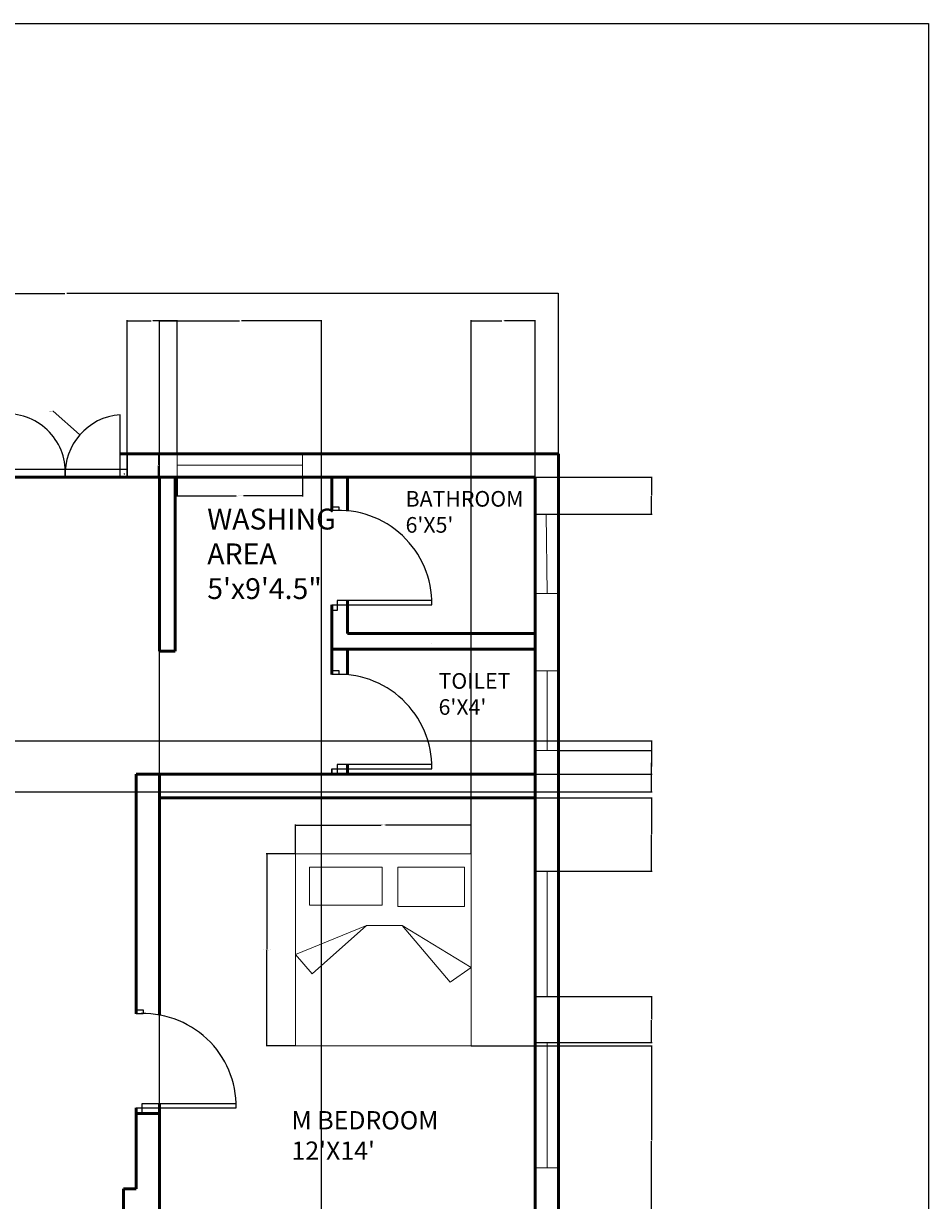
# Model space of a CAD drawing. Units: inches. Extents: x -177 to 2564, y -706 to 2548.
# Tile 4 of 4: x 176 to 523, y -266 to 186. Entities that reach past the tile are written whole.
import ezdxf

# ---------------------------------------------------------------- set-up
doc = ezdxf.new("R2010")
doc.units = ezdxf.units.IN
doc.header["$MEASUREMENT"] = 0
for name, color, linetype, lineweight in [('A-ANNO-DIMS', 2, 'Continuous', 18), ('A-ANNO-TTLB', 7, 'Continuous', 25), ('A-AREA-IDEN', 7, 'Continuous', 25), ('A-DOOR', 3, 'Continuous', 25), ('A-FURN', 8, 'Continuous', 18), ('A-GLAZ', 4, 'Continuous', 18), ('A-WALL', 7, 'Continuous', 50)]:
    doc.layers.add(name, color=color, linetype=linetype, lineweight=lineweight)
doc.styles.get("Standard").update_dxf_attribs({"font": 'arial.ttf'})
doc.dimstyles.get("Standard").update_dxf_attribs({"dimtxt": 0.18, "dimasz": 0.18, "dimexe": 0.18, "dimexo": 0.0625, "dimgap": 0.09, "dimtad": 0, "dimtih": 1, "dimtoh": 1, "dimdec": 0, "dimzin": 0, "dimdsep": 46, "dimlunit": 4, "dimtxsty": 'Standard', "dimcen": 0.09, "dimadec": 0, "dimazin": 0, "dimtfac": 1, "dimtdec": 0, "dimtofl": 0, "dimtmove": 0, "dimatfit": 3, "dimfxl": 1, "dimtolj": 1, "dimtzin": 0, "dimarcsym": 0})

# ---------------------------------------------------------------- blocks, each defined once
blk = doc.blocks.new('*D1')
at = {"layer": 'A-ANNO-DIMS', "color": 0, "lineweight": -2, "transparency": 16777216}
for p, q in [((3.47, 20.6), (3.47, 82.15)), ((3.65, 81.97), (192.07, 81.97)), ((381.29, 81.97), (192.87, 81.97)), ((381.47, 20.6), (381.47, 82.15))]:
    blk.add_line(p, q, dxfattribs=at)
at = {"layer": 'A-ANNO-DIMS', "color": 0, "transparency": 16777216}
for points in [[(3.65, 82), (3.65, 81.94), (3.47, 81.97)], [(381.29, 82), (381.29, 81.94), (381.47, 81.97)]]:
    blk.add_solid(points, dxfattribs=at)
at = {"layer": 'Defpoints', "color": 0, "transparency": 16777216}
for p in [(381.47, 81.97), (3.47, 20.54), (381.47, 20.54)]:
    blk.add_point(p, dxfattribs=at)
at = {"layer": 'A-ANNO-DIMS', "color": 0, "transparency": 16777216, "insert": (192.47, 81.97), "char_height": 0.18, "attachment_point": 5}
blk.add_mtext('\\A1;31\'-6"', dxfattribs=at)
blk = doc.blocks.new('BED-DOUBLE')
for p, q in [((0, -38.58), (27.19, -27.51)), ((27.19, -27.51), (6.3, -46)), ((27.19, -27.51), (40.92, -27.51)), ((40.92, -27.51), (27.19, -27.51)), ((40.92, -27.51), (67.3, -43.62)), ((59.29, -49.22), (40.92, -27.51)), ((0, -73.65), (0, -38.58)), ((6.3, -46), (0, -38.58)), ((67.3, -43.62), (59.29, -49.22))]:
    blk.add_line(p, q)
for points in [[(0, 0), (67.3, 0), (67.3, -73.65), (0, -73.65)], [(5.32, -5.1), (33.21, -5.1), (33.21, -19.67), (5.32, -19.67)], [(39.24, -5.1), (64.75, -5.1), (64.75, -20.23), (39.24, -20.23)]]:
    blk.add_lwpolyline(points, close=True)
blk = doc.blocks.new('WIN-48')
for p, q in [((0, 0), (9, 0)), ((9, 0), (4.59, 0)), ((4.59, 0), (4.59, -48.06)), ((9, -48.06), (0, -48.06))]:
    blk.add_line(p, q)
blk = doc.blocks.new('WIN-30')
for p, q in [((0, 30.54), (-9, 30.54)), ((-4.41, 0), (-4.41, 30.54)), ((0, 0), (-9, 0)), ((0, 0), (-4.41, 0))]:
    blk.add_line(p, q)
blk = doc.blocks.new('DOOR-SINGLE-36')
for p, q in [((1.57, 36.24), (0, 36.24)), ((0, 36.24), (0, 0)), ((1.57, -2.14), (1.57, 36.24)), ((1.57, 36.24), (1.57, 36.24)), ((-36.05, -2.14), (-36.05, 0.59)), ((-36.05, 0.59), (-34.54, 0.59)), ((-34.54, 0.59), (-34.54, -2.14)), ((0, 0), (3.72, 0)), ((3.72, 0), (3.72, -2.14)), ((3.72, -2.14), (1.57, -2.14))]:
    blk.add_line(p, q)
blk.add_arc((1.05, 0.56), 35.69, 89.1597, 184.3396)
blk = doc.blocks.new('DOOR-PAIR-44')
for p, q in [((0, 0), (0, 24.32)), ((44.01, 0), (44.01, 23.95)), ((-2.88, 0), (-2.88, 3.11)), ((-2.88, 3.11), (46.72, 3.11)), ((46.72, 0), (-2.88, 0)), ((-2.88, 0), (0, 0)), ((0, 0), (44.01, 0)), ((23.01, 0), (23.01, 3.55)), ((44.01, 0), (23.01, 0)), ((46.72, 0), (44.01, 0))]:
    blk.add_line(p, q)
for centre, radius, start, end in [((0.52, 1.77), 22.55, 355.4915, 91.326), ((45.7, 1.28), 22.73, 94.2755, 183.2347)]:
    blk.add_arc(centre, radius, start, end)
blk = doc.blocks.new('*D10')
at = {"layer": 'A-ANNO-DIMS', "color": 0, "lineweight": -2, "transparency": 16777216}
for p, q in [((235.2, 11.47), (235.2, 4.15)), ((283.26, 11.47), (283.26, 4.15)), ((235.38, 4.33), (257.78, 4.33)), ((283.08, 4.33), (260.68, 4.33))]:
    blk.add_line(p, q, dxfattribs=at)
at = {"layer": 'A-ANNO-DIMS', "color": 0, "transparency": 16777216}
for points in [[(235.38, 4.36), (235.38, 4.3), (235.2, 4.33)], [(283.08, 4.36), (283.08, 4.3), (283.26, 4.33)]]:
    blk.add_solid(points, dxfattribs=at)
at = {"layer": 'Defpoints', "color": 0, "transparency": 16777216}
for p in [(235.2, 11.54), (283.26, 11.54), (235.2, 4.33)]:
    blk.add_point(p, dxfattribs=at)
at = {"layer": 'A-ANNO-DIMS', "color": 0, "transparency": 16777216, "insert": (259.23, 4.33), "char_height": 0.18, "attachment_point": 5}
blk.add_mtext('\\A1;WINDOW W1 4\'-0" TYP.', dxfattribs=at)
blk = doc.blocks.new('*D11')
at = {"layer": 'A-ANNO-DIMS', "color": 0, "lineweight": -2, "transparency": 16777216}
for p, q in [((235.14, 20.54), (227.81, 20.54)), ((227.99, 20.36), (227.99, 16.22)), ((227.99, 11.72), (227.99, 15.85)), ((235.14, 11.54), (227.81, 11.54))]:
    blk.add_line(p, q, dxfattribs=at)
at = {"layer": 'A-ANNO-DIMS', "color": 0, "transparency": 16777216}
for points in [[(227.96, 20.36), (228.02, 20.36), (227.99, 20.54)], [(227.96, 11.72), (228.02, 11.72), (227.99, 11.54)]]:
    blk.add_solid(points, dxfattribs=at)
at = {"layer": 'Defpoints', "color": 0, "transparency": 16777216}
for p in [(227.99, 20.54), (235.2, 20.54), (235.2, 11.54)]:
    blk.add_point(p, dxfattribs=at)
at = {"layer": 'A-ANNO-DIMS', "color": 0, "transparency": 16777216, "insert": (227.99, 16.04), "char_height": 0.18, "attachment_point": 5}
blk.add_mtext('\\A1;0\'-9" TYP.', dxfattribs=at)
blk = doc.blocks.new('*D14')
at = {"layer": 'A-ANNO-DIMS', "color": 0, "lineweight": -2, "transparency": 16777216}
for p, q in [((280.56, -132.99), (269.4, -132.99)), ((269.58, -133.17), (269.58, -169.63)), ((269.58, -206.45), (269.58, -169.99)), ((280.56, -206.63), (269.4, -206.63))]:
    blk.add_line(p, q, dxfattribs=at)
at = {"layer": 'A-ANNO-DIMS', "color": 0, "transparency": 16777216}
for points in [[(269.55, -133.17), (269.61, -133.17), (269.58, -132.99)], [(269.55, -206.45), (269.61, -206.45), (269.58, -206.63)]]:
    blk.add_solid(points, dxfattribs=at)
at = {"layer": 'Defpoints', "color": 0, "transparency": 16777216}
for p in [(269.58, -132.99), (280.63, -132.99), (280.63, -206.63)]:
    blk.add_point(p, dxfattribs=at)
at = {"layer": 'A-ANNO-DIMS', "color": 0, "transparency": 16777216, "insert": (269.58, -169.81), "char_height": 0.18, "attachment_point": 5}
blk.add_mtext('\\A1;DOUBLE BED 6\'-1 1/2" TYP.', dxfattribs=at)
blk = doc.blocks.new('*D15')
at = {"layer": 'A-ANNO-DIMS', "color": 0, "lineweight": -2, "transparency": 16777216}
for p, q in [((280.63, -132.92), (280.63, -121.76)), ((347.93, -132.92), (347.93, -121.76)), ((280.81, -121.94), (313.43, -121.94)), ((347.75, -121.94), (315.13, -121.94))]:
    blk.add_line(p, q, dxfattribs=at)
at = {"layer": 'A-ANNO-DIMS', "color": 0, "transparency": 16777216}
for points in [[(280.81, -121.91), (280.81, -121.97), (280.63, -121.94)], [(347.75, -121.91), (347.75, -121.97), (347.93, -121.94)]]:
    blk.add_solid(points, dxfattribs=at)
at = {"layer": 'Defpoints', "color": 0, "transparency": 16777216}
for p in [(347.93, -121.94), (280.63, -132.99), (347.93, -132.99)]:
    blk.add_point(p, dxfattribs=at)
at = {"layer": 'A-ANNO-DIMS', "color": 0, "transparency": 16777216, "insert": (314.28, -121.94), "char_height": 0.18, "attachment_point": 5}
blk.add_mtext('\\A1;5\'-7 1/2" TYP.', dxfattribs=at)
blk = doc.blocks.new('*D36')
at = {"layer": 'A-ANNO-DIMS', "color": 0, "lineweight": -2, "transparency": 16777216}
for p, q in [((41.71, -89.59), (417.35, -89.59)), ((417.17, -89.77), (417.17, -99.17)), ((417.17, -108.95), (417.17, -99.54)), ((41.71, -109.13), (417.35, -109.13))]:
    blk.add_line(p, q, dxfattribs=at)
at = {"layer": 'A-ANNO-DIMS', "color": 0, "transparency": 16777216}
for points in [[(417.14, -89.77), (417.2, -89.77), (417.17, -89.59)], [(417.14, -108.95), (417.2, -108.95), (417.17, -109.13)]]:
    blk.add_solid(points, dxfattribs=at)
at = {"layer": 'Defpoints', "color": 0, "transparency": 16777216}
for p in [(41.65, -89.59), (41.65, -109.13), (417.17, -109.13)]:
    blk.add_point(p, dxfattribs=at)
at = {"layer": 'A-ANNO-DIMS', "color": 0, "transparency": 16777216, "insert": (417.17, -99.36), "char_height": 0.18, "attachment_point": 5}
blk.add_mtext('\\A1;1\'-7 1/2"', dxfattribs=at)
blk = doc.blocks.new('*D44')
at = {"layer": 'A-ANNO-DIMS', "color": 0, "lineweight": -2, "transparency": 16777216}
for p, q in [((372.54, -111.46), (417.35, -111.46)), ((417.17, -111.64), (417.17, -125.39)), ((417.17, -139.49), (417.17, -125.75)), ((372.54, -139.67), (417.35, -139.67))]:
    blk.add_line(p, q, dxfattribs=at)
at = {"layer": 'A-ANNO-DIMS', "color": 0, "transparency": 16777216}
for points in [[(417.14, -111.64), (417.2, -111.64), (417.17, -111.46)], [(417.14, -139.49), (417.2, -139.49), (417.17, -139.67)]]:
    blk.add_solid(points, dxfattribs=at)
at = {"layer": 'Defpoints', "color": 0, "transparency": 16777216}
for p in [(372.47, -111.46), (372.47, -139.67), (417.17, -139.67)]:
    blk.add_point(p, dxfattribs=at)
at = {"layer": 'A-ANNO-DIMS', "color": 0, "transparency": 16777216, "insert": (417.17, -125.57), "char_height": 0.18, "attachment_point": 5}
blk.add_mtext('\\A1;2\'-4"', dxfattribs=at)
blk = doc.blocks.new('*D45')
at = {"layer": 'A-ANNO-DIMS', "color": 0, "lineweight": -2, "transparency": 16777216}
for p, q in [((372.54, -187.73), (417.35, -187.73)), ((417.17, -187.91), (417.17, -196.38)), ((417.17, -205.22), (417.17, -196.75)), ((372.54, -205.4), (417.35, -205.4))]:
    blk.add_line(p, q, dxfattribs=at)
at = {"layer": 'A-ANNO-DIMS', "color": 0, "transparency": 16777216}
for points in [[(417.14, -187.91), (417.2, -187.91), (417.17, -187.73)], [(417.14, -205.22), (417.2, -205.22), (417.17, -205.4)]]:
    blk.add_solid(points, dxfattribs=at)
at = {"layer": 'Defpoints', "color": 0, "transparency": 16777216}
for p in [(372.47, -187.73), (372.47, -205.4), (417.17, -205.4)]:
    blk.add_point(p, dxfattribs=at)
at = {"layer": 'A-ANNO-DIMS', "color": 0, "transparency": 16777216, "insert": (417.17, -196.56), "char_height": 0.18, "attachment_point": 5}
blk.add_mtext('\\A1;1\'-5 1/2"', dxfattribs=at)
blk = doc.blocks.new('*D46')
at = {"layer": 'A-ANNO-DIMS', "color": 0, "lineweight": -2, "transparency": 16777216}
for p, q in [((347.93, -132.92), (347.93, 71.74)), ((348.11, 71.56), (359.66, 71.56)), ((372.29, 71.56), (360.74, 71.56)), ((372.47, -111.4), (372.47, 71.74))]:
    blk.add_line(p, q, dxfattribs=at)
at = {"layer": 'A-ANNO-DIMS', "color": 0, "transparency": 16777216}
for points in [[(348.11, 71.59), (348.11, 71.53), (347.93, 71.56)], [(372.29, 71.59), (372.29, 71.53), (372.47, 71.56)]]:
    blk.add_solid(points, dxfattribs=at)
at = {"layer": 'Defpoints', "color": 0, "transparency": 16777216}
for p in [(347.93, 71.56), (372.47, -111.46), (347.93, -132.99)]:
    blk.add_point(p, dxfattribs=at)
at = {"layer": 'A-ANNO-DIMS', "color": 0, "transparency": 16777216, "insert": (360.2, 71.56), "char_height": 0.18, "attachment_point": 5}
blk.add_mtext('\\A1;2\'-0 1/2"', dxfattribs=at)
blk = doc.blocks.new('*D47')
at = {"layer": 'A-ANNO-DIMS', "color": 0, "lineweight": -2, "transparency": 16777216}
for p, q in [((347.99, -206.63), (417.35, -206.63)), ((417.17, -206.81), (417.17, -242.87)), ((417.17, -279.28), (417.17, -243.23)), ((372.54, -279.46), (417.35, -279.46))]:
    blk.add_line(p, q, dxfattribs=at)
at = {"layer": 'A-ANNO-DIMS', "color": 0, "transparency": 16777216}
for points in [[(417.14, -206.81), (417.2, -206.81), (417.17, -206.63)], [(417.14, -279.28), (417.2, -279.28), (417.17, -279.46)]]:
    blk.add_solid(points, dxfattribs=at)
at = {"layer": 'Defpoints', "color": 0, "transparency": 16777216}
for p in [(347.93, -206.63), (417.17, -206.63), (372.47, -279.46)]:
    blk.add_point(p, dxfattribs=at)
at = {"layer": 'A-ANNO-DIMS', "color": 0, "transparency": 16777216, "insert": (417.17, -243.05), "char_height": 0.18, "attachment_point": 5}
blk.add_mtext('\\A1;6\'-1"', dxfattribs=at)
blk = doc.blocks.new('*D48')
at = {"layer": 'A-ANNO-DIMS', "color": 0, "lineweight": -2, "transparency": 16777216}
for p, q in [((228.47, -477.4), (228.47, 71.74)), ((228.65, 71.56), (259.17, 71.56)), ((290.34, 71.56), (259.83, 71.56)), ((290.52, -443.93), (290.52, 71.74))]:
    blk.add_line(p, q, dxfattribs=at)
at = {"layer": 'A-ANNO-DIMS', "color": 0, "transparency": 16777216}
for points in [[(228.65, 71.59), (228.65, 71.53), (228.47, 71.56)], [(290.34, 71.59), (290.34, 71.53), (290.52, 71.56)]]:
    blk.add_solid(points, dxfattribs=at)
at = {"layer": 'Defpoints', "color": 0, "transparency": 16777216}
for p in [(290.52, 71.56), (290.52, -443.99), (228.47, -477.46)]:
    blk.add_point(p, dxfattribs=at)
at = {"layer": 'A-ANNO-DIMS', "color": 0, "transparency": 16777216, "insert": (259.5, 71.56), "char_height": 0.18, "attachment_point": 5}
blk.add_mtext('\\A1;5\'-2"', dxfattribs=at)
blk = doc.blocks.new('*D52')
at = {"layer": 'A-ANNO-DIMS', "color": 0, "lineweight": -2, "transparency": 16777216}
for p, q in [((216.02, 20.6), (216.02, 71.74)), ((216.2, 71.56), (225.29, 71.56)), ((235.02, 71.56), (225.93, 71.56)), ((235.2, 20.6), (235.2, 71.74))]:
    blk.add_line(p, q, dxfattribs=at)
at = {"layer": 'A-ANNO-DIMS', "color": 0, "transparency": 16777216}
for points in [[(216.2, 71.59), (216.2, 71.53), (216.02, 71.56)], [(235.02, 71.59), (235.02, 71.53), (235.2, 71.56)]]:
    blk.add_solid(points, dxfattribs=at)
at = {"layer": 'Defpoints', "color": 0, "transparency": 16777216}
for p in [(235.2, 71.56), (216.02, 20.54), (235.2, 20.54)]:
    blk.add_point(p, dxfattribs=at)
at = {"layer": 'A-ANNO-DIMS', "color": 0, "transparency": 16777216, "insert": (225.61, 71.56), "char_height": 0.18, "attachment_point": 5}
blk.add_mtext('\\A1;1\'-7"', dxfattribs=at)
blk = doc.blocks.new('*D59')
at = {"layer": 'A-ANNO-DIMS', "color": 0, "lineweight": -2, "transparency": 16777216}
for p, q in [((372.54, 11.54), (417.35, 11.54)), ((417.17, 11.36), (417.17, 4.64)), ((417.17, -2.44), (417.17, 4.28)), ((372.54, -2.62), (417.35, -2.62))]:
    blk.add_line(p, q, dxfattribs=at)
at = {"layer": 'A-ANNO-DIMS', "color": 0, "transparency": 16777216}
for points in [[(417.14, 11.36), (417.2, 11.36), (417.17, 11.54)], [(417.14, -2.44), (417.2, -2.44), (417.17, -2.62)]]:
    blk.add_solid(points, dxfattribs=at)
at = {"layer": 'Defpoints', "color": 0, "transparency": 16777216}
for p in [(372.47, 11.54), (372.47, -2.62), (417.17, -2.62)]:
    blk.add_point(p, dxfattribs=at)
at = {"layer": 'A-ANNO-DIMS', "color": 0, "transparency": 16777216, "insert": (417.17, 4.46), "char_height": 0.18, "attachment_point": 5}
blk.add_mtext('\\A1;1\'-2"', dxfattribs=at)
blk = doc.blocks.new('*D60')
at = {"layer": 'A-ANNO-DIMS', "color": 0, "lineweight": -2, "transparency": 16777216}
for p, q in [((381.54, -93.34), (417.35, -93.34)), ((417.17, -93.52), (417.17, -97.72)), ((417.17, -102.28), (417.17, -98.08)), ((372.54, -102.46), (417.35, -102.46))]:
    blk.add_line(p, q, dxfattribs=at)
at = {"layer": 'A-ANNO-DIMS', "color": 0, "transparency": 16777216}
for points in [[(417.14, -93.52), (417.2, -93.52), (417.17, -93.34)], [(417.14, -102.28), (417.2, -102.28), (417.17, -102.46)]]:
    blk.add_solid(points, dxfattribs=at)
at = {"layer": 'Defpoints', "color": 0, "transparency": 16777216}
for p in [(381.47, -93.34), (417.17, -93.34), (372.47, -102.46)]:
    blk.add_point(p, dxfattribs=at)
at = {"layer": 'A-ANNO-DIMS', "color": 0, "transparency": 16777216, "insert": (417.17, -97.9), "char_height": 0.18, "attachment_point": 5}
blk.add_mtext('\\A1;0\'-9"', dxfattribs=at)
blk = doc.blocks.new('*D64')
at = {"layer": 'A-ANNO-DIMS', "color": 0, "lineweight": -2, "transparency": 16777216}
for p, q in [((187.47, 36.8), (187.65, 36.8)), ((187.65, 36.8), (197.77, 27.92)), ((214.91, 12.82), (215.09, 12.82)), ((215, 12.73), (215, 12.91))]:
    blk.add_line(p, q, dxfattribs=at)
at = {"layer": 'A-ANNO-DIMS', "color": 0, "transparency": 16777216}
blk.add_solid([(197.79, 27.95), (197.75, 27.9), (197.91, 27.8)], dxfattribs=at)
at = {"layer": 'Defpoints', "color": 0, "transparency": 16777216}
for p in [(197.91, 27.8), (215, 12.82)]:
    blk.add_point(p, dxfattribs=at)
at = {"layer": 'A-ANNO-DIMS', "color": 0, "transparency": 16777216, "insert": (186.58, 36.8), "char_height": 0.18, "attachment_point": 5}
blk.add_mtext('\\A1;2X R1\'-10 1/2"', dxfattribs=at)

msp = doc.modelspace()

# ---------------------------------------------------------------- linework, layer by layer
at = {"layer": 'A-ANNO-TTLB'}
msp.add_lwpolyline([(-176.6, 185.58), (523.32, 185.58), (523.32, -705.52), (-176.6, -705.52)], close=True, dxfattribs=at)
at = {"layer": 'A-DOOR'}
for p, q in [((216.02, 20.54), (216.02, 11.54)), ((216.02, 11.54), (216.02, 20.54)), ((294.47, 0.21), (297.2, 0.21)), ((297.2, 0.21), (297.2, -1.2)), ((332.86, -35.84), (296.61, -35.84)), ((296.61, -35.84), (296.61, -39.56)), ((294.47, -37.41), (332.86, -37.41)), ((296.61, -39.56), (294.47, -39.56)), ((294.47, -54.46), (294.47, -52.32)), ((332.86, -52.32), (332.86, -52.32)), ((296.61, -54.46), (294.47, -54.46)), ((294.47, -62.69), (294.47, -64.21)), ((294.47, -100.32), (294.47, -102.46)), ((219.47, -192.85), (219.47, -194.37))]:
    msp.add_line(p, q, dxfattribs=at)
msp.add_arc((297.17, -36.89), 35.69, 359.1597, 94.3396, dxfattribs=at)
at = {"layer": 'A-GLAZ'}
for p, q in [((381.47, -2.62), (372.47, -2.62)), ((372.47, -2.62), (376.75, -2.62)), ((376.75, -2.62), (377.07, -33.16)), ((372.47, -33.16), (381.47, -33.16)), ((381.47, -33.16), (377.07, -33.16)), ((381.47, -93.34), (372.47, -93.34)), ((372.47, -93.34), (381.47, -93.34)), ((377.07, -139.67), (377.07, -187.73))]:
    msp.add_line(p, q, dxfattribs=at)
at = {"layer": 'A-WALL'}
for p, q in [((213.3, 20.54), (372.47, 20.54)), ((372.47, 20.54), (381.47, 20.54)), ((381.47, -601.46), (381.47, 20.54)), ((12.47, 11.54), (372.47, 11.54)), ((228.47, 11.54), (216.02, 11.54)), ((228.47, -55.18), (228.47, 11.54)), ((294.47, 11.54), (234.47, 11.54)), ((234.47, 11.54), (234.47, -55.18)), ((294.47, -1.3), (294.47, 11.54)), ((372.47, 11.54), (300.47, 11.54)), ((300.47, 11.54), (300.47, -1.35)), ((372.47, 11.54), (372.47, -601.46)), ((300.47, -35.84), (300.47, -48.46)), ((294.47, -54.46), (294.47, -37.41)), ((294.47, -37.41), (294.47, -52.32)), ((300.47, -48.46), (372.47, -48.46)), ((372.47, -48.46), (372.47, -54.46)), ((234.47, -55.18), (228.47, -55.18)), ((300.47, -54.46), (294.47, -54.46)), ((366.47, -54.46), (294.47, -54.46)), ((294.47, -54.46), (294.47, -64.21)), ((372.47, -54.46), (300.47, -54.46)), ((300.47, -64.26), (300.47, -54.46)), ((372.47, -54.46), (366.47, -54.46)), ((372.47, -54.46), (372.47, -102.46)), ((300.47, -102.46), (300.47, -98.75)), ((228.47, -102.46), (219.47, -102.46)), ((219.47, -102.46), (219.47, -194.37)), ((372.47, -102.46), (228.47, -102.46)), ((228.47, -102.46), (228.47, -111.46)), ((294.47, -102.46), (300.47, -102.46)), ((228.47, -111.46), (372.47, -111.46)), ((228.47, -111.46), (228.47, -194.82)), ((228.47, -228.9), (228.47, -279.46)), ((219.47, -230.47), (219.47, -261.46)), ((219.47, -232.62), (228.47, -232.62)), ((219.47, -261.46), (219.47, -232.62)), ((214.58, -270.46), (214.58, -261.46)), ((214.58, -261.46), (219.47, -261.46))]:
    msp.add_line(p, q, dxfattribs=at)

# ---------------------------------------------------------------- block references
at = {"layer": 'A-DOOR'}
msp.add_blockref('DOOR-PAIR-44', (169.3, 11.54), dxfattribs=at)
for p, rotation in [((296.61, -98.75), 270.0000000000002), ((221.61, -228.9), 270)]:
    msp.add_blockref('DOOR-SINGLE-36', p, dxfattribs=dict(at, rotation=rotation))
at = {"layer": 'A-FURN'}
msp.add_blockref('BED-DOUBLE', (280.63, -132.99), dxfattribs=at)
at = {"layer": 'A-GLAZ', "rotation": 89.99999999999984}
msp.add_blockref('WIN-48', (235.2, 11.54), dxfattribs=at)
at = {"layer": 'A-GLAZ'}
for name, p in [('WIN-30', (381.47, -93.34)), ('WIN-48', (372.47, -139.67)), ('WIN-48', (372.47, -205.4))]:
    msp.add_blockref(name, p, dxfattribs=at)

# ---------------------------------------------------------------- texts
at = {"layer": 'A-AREA-IDEN', "attachment_point": 1}
for s, insert, char_height in [("BATHROOM\\P6'X5'", (322.8, 6.23), 6), ('WASHING\\PAREA\\P5\'x9\'4.5"', (246.74, -0.55), 8), ("M BEDROOM\\P12'X14'", (279.05, -231.69), 7)]:
    msp.add_mtext(s, dxfattribs=dict(at, insert=insert, char_height=char_height))
at = {"layer": 'A-AREA-IDEN', "insert": (335.45, -63.64), "char_height": 6, "attachment_point": 1}
msp.add_mtext_dynamic_manual_height_columns("TOILET\\P6'X4'", width=29.3378, gutter_width=1, heights=[0], dxfattribs=at)

# ---------------------------------------------------------------- dimensions: what is measured, and where the dimension line sits
at = {"layer": 'A-ANNO-DIMS'}
for base, p1, p2, override, picture, middle in [((381.47, 81.97), (3.47, 20.54), (381.47, 20.54), {"dimclrd": 0, "dimclre": 0, "dimclrt": 0}, '*D1', (192.47, 81.97)), ((235.2, 71.56), (216.02, 20.54), (235.2, 20.54), {"dimdec": 1, "dimlfac": 1, "dimrnd": 0, "dimzin": 1, "dimdsep": 46, "dimlunit": 4, "dimfrac": 2}, '*D52', (225.61, 71.56)), ((290.52, 71.5552), (228.4733, -477.4645), (290.52, -443.9906), {"dimdec": 1, "dimlfac": 1, "dimrnd": 0, "dimzin": 1, "dimdsep": 46, "dimlunit": 4, "dimfrac": 2}, '*D48', (259.4967, 71.5552)), ((347.93, 71.56), (372.47, -111.46), (347.93, -132.99), {"dimdec": 1, "dimlfac": 1, "dimrnd": 0, "dimzin": 1, "dimdsep": 46, "dimlunit": 4, "dimfrac": 2}, '*D46', (360.2, 71.56))]:
    dim = msp.add_linear_dim(base=base, p1=p1, p2=p2, dimstyle='Standard', override=override, dxfattribs=at)
    dim.commit()
    dim.dimension.update_dxf_attribs({"geometry": picture, "text_midpoint": middle})
dim = msp.add_radius_dim(center=(215, 12.82), mpoint=(197.91, 27.8), text='2X <>', dimstyle='Standard', override={"dimdec": 1, "dimlfac": 1, "dimrnd": 0, "dimzin": 1, "dimdsep": 46, "dimlunit": 4, "dimfrac": 2}, dxfattribs=at)
dim.commit()
dim.dimension.update_dxf_attribs({"geometry": '*D64', "text_midpoint": (186.58, 36.8), "dimtype": 164})
for base, p1, p2, angle, text, picture, middle in [((227.99, 20.54), (235.2, 11.54), (235.2, 20.54), 90, '<> TYP.', '*D11', (227.99, 16.04)), ((235.2, 4.33), (283.26, 11.54), (235.2, 11.54), 180, 'WINDOW W1 <> TYP.', '*D10', (259.23, 4.33)), ((269.58, -132.99), (280.63, -206.63), (280.63, -132.99), 90, 'DOUBLE BED <> TYP.', '*D14', (269.58, -169.81))]:
    dim = msp.add_linear_dim(base=base, p1=p1, p2=p2, angle=angle, text=text, dimstyle='Standard', override={"dimdec": 1, "dimlfac": 1, "dimrnd": 0, "dimzin": 1, "dimdsep": 46, "dimlunit": 4, "dimfrac": 2}, dxfattribs=at)
    dim.commit()
    dim.dimension.update_dxf_attribs({"geometry": picture, "text_midpoint": middle})
for base, p1, p2, picture, middle in [((417.17, -2.62), (372.47, 11.54), (372.47, -2.62), '*D59', (417.17, 4.46)), ((417.17, -109.13), (41.65, -89.59), (41.65, -109.13), '*D36', (417.17, -99.36)), ((417.17, -93.34), (372.47, -102.46), (381.47, -93.34), '*D60', (417.17, -97.9)), ((417.17, -139.67), (372.47, -111.46), (372.47, -139.67), '*D44', (417.17, -125.57)), ((417.17, -205.4), (372.47, -187.73), (372.47, -205.4), '*D45', (417.17, -196.56)), ((417.17, -206.63), (372.47, -279.46), (347.93, -206.63), '*D47', (417.17, -243.05))]:
    dim = msp.add_linear_dim(base=base, p1=p1, p2=p2, angle=90, dimstyle='Standard', override={"dimdec": 1, "dimlfac": 1, "dimrnd": 0, "dimzin": 1, "dimdsep": 46, "dimlunit": 4, "dimfrac": 2}, dxfattribs=at)
    dim.commit()
    dim.dimension.update_dxf_attribs({"geometry": picture, "text_midpoint": middle})
dim = msp.add_linear_dim(base=(347.93, -121.94), p1=(280.63, -132.99), p2=(347.93, -132.99), text='<> TYP.', dimstyle='Standard', override={"dimdec": 1, "dimlfac": 1, "dimrnd": 0, "dimzin": 1, "dimdsep": 46, "dimlunit": 4, "dimfrac": 2}, dxfattribs=at)
dim.commit()
dim.dimension.update_dxf_attribs({"geometry": '*D15', "text_midpoint": (314.28, -121.94)})

doc.saveas('drawing.dxf')
